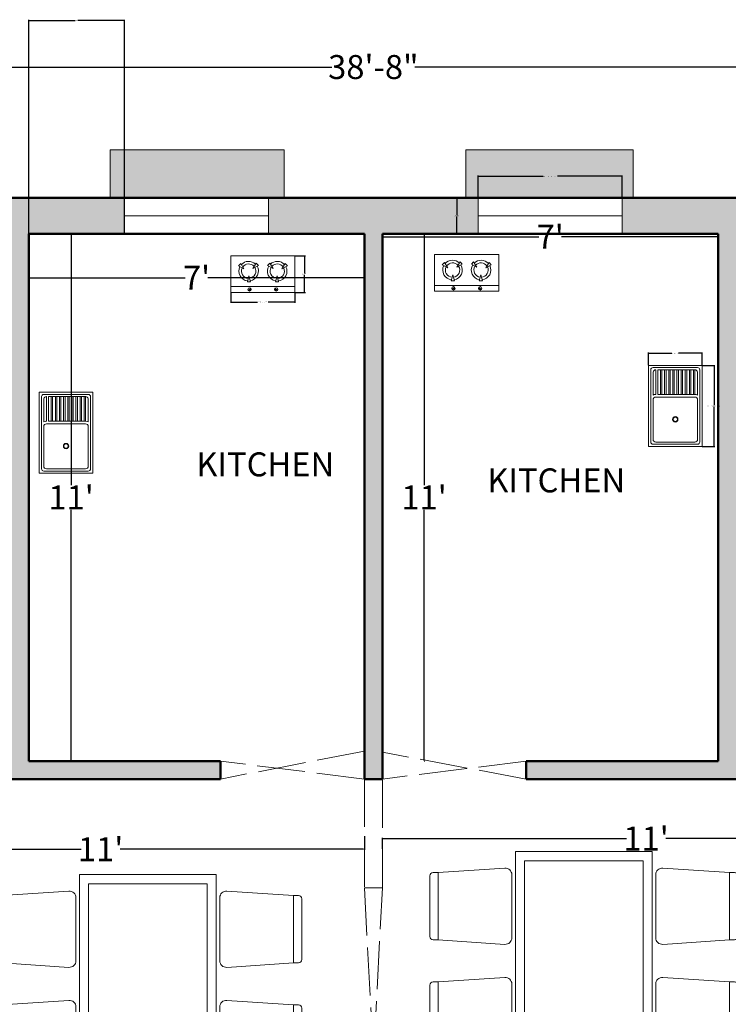
# Model space of a CAD drawing. Units: inches. Extents: x -28 to 544, y -640 to 52.
# Tile 8 of 11: x 160 to 338, y -194 to 52. Entities that reach past the tile are written whole.
import ezdxf

# ---------------------------------------------------------------- set-up
doc = ezdxf.new("R2010")
doc.units = ezdxf.units.IN
doc.header["$MEASUREMENT"] = 0
doc.linetypes.add('ACAD_ISO02W100', pattern=[15, 12, -3])
for name, color, linetype, lineweight in [('A-ANNO-DIMS', 2, 'Continuous', 18), ('A-AREA-IDEN', 7, 'Continuous', 25), ('A-EQPM', 8, 'Continuous', 18), ('A-FLOR-FIXT', 9, 'Continuous', 20), ('A-FURN', 8, 'Continuous', 18), ('A-GLAZ', 4, 'Continuous', 20), ('A-ROOF', 8, 'Continuous', 18), ('A-ROOF-PATT', 252, 'Continuous', 13), ('A-WALL', 7, 'Continuous', 50), ('A-WALL-OVHD', 8, 'ACAD_ISO02W100', 18), ('A-WALL-PATT', 5, 'Continuous', 13)]:
    doc.layers.add(name, color=color, linetype=linetype, lineweight=lineweight)
doc.styles.get("Standard").update_dxf_attribs({"font": 'arial.ttf'})
doc.dimstyles.get("Standard").update_dxf_attribs({"dimtxt": 0.18, "dimasz": 0.18, "dimexe": 0.18, "dimexo": 0.0625, "dimgap": 0.09, "dimtad": 0, "dimtih": 1, "dimtoh": 1, "dimdec": 0, "dimzin": 0, "dimdsep": 46, "dimlunit": 3, "dimtxsty": 'Standard', "dimcen": 0.09, "dimadec": 0, "dimazin": 0, "dimtfac": 1, "dimtdec": 0, "dimtofl": 0, "dimtmove": 0, "dimatfit": 3, "dimfxl": 1, "dimtolj": 1, "dimtzin": 0, "dimarcsym": 0})

# ---------------------------------------------------------------- blocks, each defined once
blk = doc.blocks.new('*D3')
at = {"layer": 'A-ANNO-DIMS', "color": 0, "lineweight": -2, "transparency": 16777216}
for p, q in [((173.13, -1.24), (172.89, -1.24)), ((173.07, -1.42), (173.07, -64.14)), ((173.07, -133.06), (173.07, -70.34)), ((173.13, -133.24), (172.89, -133.24))]:
    blk.add_line(p, q, dxfattribs=at)
at = {"layer": 'A-ANNO-DIMS', "color": 0, "transparency": 16777216}
for points in [[(173.04, -1.42), (173.1, -1.42), (173.07, -1.24)], [(173.04, -133.06), (173.1, -133.06), (173.07, -133.24)]]:
    blk.add_solid(points, dxfattribs=at)
at = {"layer": 'Defpoints', "color": 0, "transparency": 16777216}
for p in [(173.19, -1.24), (173.07, -133.24), (173.19, -133.24)]:
    blk.add_point(p, dxfattribs=at)
at = {"layer": 'A-ANNO-DIMS', "color": 0, "transparency": 16777216, "insert": (173.07, -67.24), "char_height": 6, "attachment_point": 5}
blk.add_mtext("\\A1;11'", dxfattribs=at)
blk = doc.blocks.new('*D4')
at = {"layer": 'A-ANNO-DIMS', "color": 0, "lineweight": -2, "transparency": 16777216}
for p, q in [((162.44, -12.17), (162.44, -12.06)), ((162.62, -12.24), (201.62, -12.24)), ((246.26, -12.24), (207.27, -12.24)), ((246.44, -12.17), (246.44, -12.06))]:
    blk.add_line(p, q, dxfattribs=at)
at = {"layer": 'A-ANNO-DIMS', "color": 0, "transparency": 16777216}
for points in [[(162.62, -12.21), (162.62, -12.27), (162.44, -12.24)], [(246.26, -12.21), (246.26, -12.27), (246.44, -12.24)]]:
    blk.add_solid(points, dxfattribs=at)
at = {"layer": 'Defpoints', "color": 0, "transparency": 16777216}
for p in [(162.44, -12.24), (246.44, -12.24), (246.44, -12.24)]:
    blk.add_point(p, dxfattribs=at)
at = {"layer": 'A-ANNO-DIMS', "color": 0, "transparency": 16777216, "insert": (204.44, -12.24), "char_height": 6, "attachment_point": 5}
blk.add_mtext("\\A1;7'", dxfattribs=at)
blk = doc.blocks.new('*D5')
at = {"layer": 'A-ANNO-DIMS', "color": 0, "lineweight": -2, "transparency": 16777216}
for p, q in [((250.94, -3.78), (250.94, -1.8)), ((251.12, -1.98), (290.12, -1.98)), ((334.76, -1.98), (295.77, -1.98)), ((334.94, -3.78), (334.94, -1.8))]:
    blk.add_line(p, q, dxfattribs=at)
at = {"layer": 'A-ANNO-DIMS', "color": 0, "transparency": 16777216}
for points in [[(251.12, -1.95), (251.12, -2.01), (250.94, -1.98)], [(334.76, -1.95), (334.76, -2.01), (334.94, -1.98)]]:
    blk.add_solid(points, dxfattribs=at)
at = {"layer": 'Defpoints', "color": 0, "transparency": 16777216}
for p in [(334.94, -1.98), (250.94, -3.84), (334.94, -3.84)]:
    blk.add_point(p, dxfattribs=at)
at = {"layer": 'A-ANNO-DIMS', "color": 0, "transparency": 16777216, "insert": (292.94, -1.98), "char_height": 6, "attachment_point": 5}
blk.add_mtext("\\A1;7'", dxfattribs=at)
blk = doc.blocks.new('*D6')
at = {"layer": 'A-ANNO-DIMS', "color": 0, "lineweight": -2, "transparency": 16777216}
for p, q in [((261.39, -1.42), (261.39, -64.14)), ((261.45, -1.24), (261.57, -1.24)), ((261.39, -133.06), (261.39, -70.34)), ((261.45, -133.24), (261.57, -133.24))]:
    blk.add_line(p, q, dxfattribs=at)
at = {"layer": 'A-ANNO-DIMS', "color": 0, "transparency": 16777216}
for points in [[(261.36, -1.42), (261.42, -1.42), (261.39, -1.24)], [(261.36, -133.06), (261.42, -133.06), (261.39, -133.24)]]:
    blk.add_solid(points, dxfattribs=at)
at = {"layer": 'Defpoints', "color": 0, "transparency": 16777216}
for p in [(261.39, -1.24), (261.39, -133.24), (261.39, -133.24)]:
    blk.add_point(p, dxfattribs=at)
at = {"layer": 'A-ANNO-DIMS', "color": 0, "transparency": 16777216, "insert": (261.39, -67.24), "char_height": 6, "attachment_point": 5}
blk.add_mtext("\\A1;11'", dxfattribs=at)
blk = doc.blocks.new('М12 540х820')
for p, q in [((0, 540), (-820, 540)), ((-820, 540), (-820, 0)), ((-45, 517.5), (-775, 517.5)), ((0, 0), (0, 540)), ((-797.5, 495), (-797.5, 45)), ((-775, 468), (-775, 72)), ((-347.5, 495), (-748, 495)), ((-320.5, 468), (-320.5, 72)), ((-301.7, 495), (-64.8, 495)), ((-293.7, 468), (-293.7, 472.5)), ((-293.7, 468), (-45, 468)), ((-293.7, 446.6), (-45, 446.6)), ((-293.7, 419.6), (-293.7, 446.6)), ((-293.7, 419.6), (-45, 419.6)), ((-293.7, 405), (-45, 405)), ((-293.7, 378), (-293.7, 405)), ((-45, 469.5), (-45, 468)), ((-45, 419.6), (-45, 446.6)), ((-45, 378), (-45, 405)), ((-22.5, 45), (-22.5, 495)), ((-293.7, 378), (-45, 378)), ((-293.7, 336.4), (-293.7, 363.4)), ((-293.7, 363.4), (-45, 363.4)), ((-293.7, 336.4), (-45, 336.4)), ((-293.7, 294.7), (-293.7, 321.7)), ((-293.7, 321.7), (-45, 321.7)), ((-45, 336.4), (-45, 363.4)), ((-45, 294.7), (-45, 321.7)), ((-293.7, 294.7), (-45, 294.7)), ((-293.7, 253.1), (-293.7, 280.1)), ((-293.7, 280.1), (-45, 280.1)), ((-293.7, 253.1), (-45, 253.1)), ((-293.7, 211.5), (-293.7, 238.5)), ((-293.7, 238.5), (-45, 238.5)), ((-293.7, 211.5), (-45, 211.5)), ((-45, 253.1), (-45, 280.1)), ((-45, 211.5), (-45, 238.5)), ((-293.7, 169.9), (-293.7, 196.9)), ((-293.7, 196.9), (-45, 196.9)), ((-293.7, 169.9), (-45, 169.9)), ((-293.7, 128.2), (-293.7, 155.2)), ((-293.7, 155.2), (-45, 155.2)), ((-293.7, 128.2), (-45, 128.2)), ((-293.7, 113.6), (-45, 113.6)), ((-293.7, 86.6), (-293.7, 113.6)), ((-45, 169.9), (-45, 196.9)), ((-45, 128.2), (-45, 155.2)), ((-45, 86.6), (-45, 113.6)), ((-820, 0), (0, 0)), ((-775, 22.5), (-45, 22.5)), ((-748, 45), (-347.5, 45)), ((-301.7, 45), (-64.8, 45)), ((-293.7, 86.6), (-45, 86.6)), ((-293.7, 72), (-45, 72)), ((-45, 70.5), (-45, 72))]:
    blk.add_line(p, q)
at = {"ltscale": 0.06}
for p, q in [((-820, 0), (-820, 540)), ((-820, 540), (0, 540)), ((0, 540), (0, 536.9)), ((0, 536.9), (0, 0)), ((-293.7, 446.6), (-45, 446.6)), ((-293.7, 405), (-293.7, 446.6)), ((-293.7, 363.4), (-293.7, 405)), ((-45, 446.6), (-45, 419.6)), ((-45, 419.6), (-45, 378)), ((-293.7, 321.7), (-293.7, 363.4)), ((-293.7, 280.1), (-293.7, 321.7)), ((-45, 378), (-45, 336.4)), ((-45, 336.4), (-45, 294.7)), ((-293.7, 238.5), (-293.7, 280.1)), ((-293.7, 196.9), (-293.7, 238.5)), ((-45, 294.7), (-45, 253.1)), ((-45, 253.1), (-45, 211.5)), ((-45, 211.5), (-45, 169.9)), ((-293.7, 155.2), (-293.7, 196.9)), ((-293.7, 113.6), (-293.7, 155.2)), ((-293.7, 72), (-293.7, 113.6)), ((-45, 169.9), (-45, 128.2)), ((-45, 128.2), (-45, 86.6)), ((0, 0), (-820, 0)), ((-45, 72), (-293.7, 72)), ((-45, 86.6), (-45, 72))]:
    blk.add_line(p, q, dxfattribs=at)
at = {"extrusion": (0, 0, -1)}
for centre, major_axis, start_param, end_param in [((-775, 495), (-15.9, 15.9), -0.785398, 0.785398), ((-775, 495), (-15.9, 15.9), -0.785398, 0.785398), ((-45, 495), (-15.9, -15.9), 2.356194, 3.926991), ((-45, 495), (-15.9, -15.9), 2.356194, 3.926991), ((-748, 468), (-19.1, -19.1), 0.785398, 2.356194), ((-748, 468), (-19.1, -19.1), 0.785398, 2.356194), ((-347.5, 468), (-19.1, 19.1), 0.785398, 2.356194), ((-347.5, 468), (-19.1, 19.1), 0.785398, 2.356194), ((-343.2, 468), (-35, 35), 1.779263, 2.356194), ((-343.2, 468), (-35, 35), 1.779263, 2.356192), ((-343.2, 468), (-35, 35), 2.356192, 2.356194), ((-72.3, 468.8), (-19.3, 19.3), 1.0328, 2.38382), ((-72.3, 468.8), (-19.3, 19.3), 1.0328, 1.064673), ((-72.3, 468.8), (-19.3, 19.3), 1.064673, 2.328569), ((-72.3, 468.8), (-19.3, 19.3), 2.328569, 2.38382), ((-545.5, 270), (-19.1, -19.1), 3.926991, 10.210176), ((-545.5, 270), (-19.1, -19.1), 3.926991, 10.210176), ((-545.5, 270), (-15.9, -15.9), 3.926991, 10.210176), ((-545.5, 270), (-15.9, -15.9), 3.926991, 10.210176), ((-775, 45), (-15.9, -15.9), 5.497787, 7.068583), ((-775, 45), (-15.9, -15.9), 5.497787, 7.068583), ((-748, 72), (-19.1, 19.1), 3.926991, 5.497787), ((-748, 72), (-19.1, 19.1), 3.926991, 5.497787), ((-347.5, 72), (-19.1, -19.1), 3.926991, 5.497787), ((-347.5, 72), (-19.1, -19.1), 3.926991, 5.497787), ((-343.2, 72), (-35, -35), 3.926991, 4.503922), ((-343.2, 72), (-35, -35), 3.926991, 4.503922), ((-72.3, 71.2), (-19.3, -19.3), 3.899365, 5.250385), ((-72.3, 71.2), (-19.3, -19.3), 5.218512, 5.250385), ((-72.3, 71.2), (-19.3, -19.3), 3.954617, 5.218512), ((-72.3, 71.2), (-19.3, -19.3), 3.899365, 3.954617), ((-45, 45), (-15.9, 15.9), 2.356194, 3.926991), ((-45, 45), (-15.9, 15.9), 2.356194, 3.926991)]:
    blk.add_ellipse(centre, major_axis=major_axis, ratio=1, start_param=start_param, end_param=end_param, dxfattribs=at)
blk = doc.blocks.new('*D27')
at = {"layer": 'A-ANNO-DIMS', "color": 0, "lineweight": -2, "transparency": 16777216}
for p, q in [((16.94, 7.82), (16.94, 40.69)), ((17.12, 40.51), (238.3, 40.51)), ((480.26, 40.51), (259.09, 40.51)), ((480.44, 7.82), (480.44, 40.69))]:
    blk.add_line(p, q, dxfattribs=at)
at = {"layer": 'A-ANNO-DIMS', "color": 0, "transparency": 16777216}
for points in [[(17.12, 40.54), (17.12, 40.48), (16.94, 40.51)], [(480.26, 40.54), (480.26, 40.48), (480.44, 40.51)]]:
    blk.add_solid(points, dxfattribs=at)
at = {"layer": 'Defpoints', "color": 0, "transparency": 16777216}
for p in [(480.44, 40.51), (16.94, 7.76), (480.44, 7.76)]:
    blk.add_point(p, dxfattribs=at)
at = {"layer": 'A-ANNO-DIMS', "color": 0, "transparency": 16777216, "insert": (248.69, 40.51), "char_height": 6, "attachment_point": 5}
blk.add_mtext('\\A1;38\'-8"', dxfattribs=at)
blk = doc.blocks.new('*D37')
at = {"layer": 'A-ANNO-DIMS', "color": 0, "lineweight": -2, "transparency": 16777216}
for p, q in [((114.44, -152.03), (114.44, -155.48)), ((246.44, -152.03), (246.44, -155.48)), ((114.62, -155.3), (175.55, -155.3)), ((246.26, -155.3), (185.34, -155.3))]:
    blk.add_line(p, q, dxfattribs=at)
at = {"layer": 'A-ANNO-DIMS', "color": 0, "transparency": 16777216}
for points in [[(114.62, -155.27), (114.62, -155.33), (114.44, -155.3)], [(246.26, -155.27), (246.26, -155.33), (246.44, -155.3)]]:
    blk.add_solid(points, dxfattribs=at)
at = {"layer": 'Defpoints', "color": 0, "transparency": 16777216}
for p in [(114.44, -151.97), (246.44, -151.97), (246.44, -155.3)]:
    blk.add_point(p, dxfattribs=at)
at = {"layer": 'A-ANNO-DIMS', "color": 0, "transparency": 16777216, "insert": (180.44, -155.3), "char_height": 6, "attachment_point": 5}
blk.add_mtext("\\A1;11'", dxfattribs=at)
blk = doc.blocks.new('*D38')
at = {"layer": 'A-ANNO-DIMS', "color": 0, "lineweight": -2, "transparency": 16777216}
for p, q in [((250.94, -155.24), (250.94, -152.45)), ((251.12, -152.63), (312.05, -152.63)), ((382.76, -152.63), (321.84, -152.63)), ((382.94, -152.31), (382.94, -152.81))]:
    blk.add_line(p, q, dxfattribs=at)
at = {"layer": 'A-ANNO-DIMS', "color": 0, "transparency": 16777216}
for points in [[(251.12, -152.6), (251.12, -152.66), (250.94, -152.63)], [(382.76, -152.6), (382.76, -152.66), (382.94, -152.63)]]:
    blk.add_solid(points, dxfattribs=at)
at = {"layer": 'Defpoints', "color": 0, "transparency": 16777216}
for p in [(382.94, -152.25), (382.94, -152.63), (250.94, -155.3)]:
    blk.add_point(p, dxfattribs=at)
at = {"layer": 'A-ANNO-DIMS', "color": 0, "transparency": 16777216, "insert": (316.94, -152.63), "char_height": 6, "attachment_point": 5}
blk.add_mtext("\\A1;11'", dxfattribs=at)
blk = doc.blocks.new('DINING-SET-4')
for p, q in [((0.82, 49.45), (2.05, 49.45)), ((18.79, 50.59), (2.05, 49.45)), ((2.05, 32.63), (2.05, 49.45)), ((58.27, 50.59), (75.01, 49.45)), ((76.24, 49.45), (75.01, 49.45)), ((75.01, 32.63), (75.01, 49.45)), ((0, 33.45), (0, 48.63)), ((20.52, 48.95), (20.52, 33.13)), ((56.54, 48.95), (56.54, 33.13)), ((77.06, 33.45), (77.06, 48.63)), ((2.05, 32.63), (0.82, 32.63)), ((2.05, 32.63), (18.79, 31.49)), ((75.01, 32.63), (58.27, 31.49)), ((75.01, 32.63), (76.24, 32.63)), ((2.05, 22.09), (18.79, 23.23)), ((75.01, 22.09), (58.27, 23.23)), ((0, 21.27), (0, 6.09)), ((2.05, 22.09), (0.82, 22.09)), ((2.05, 22.09), (2.05, 5.27)), ((20.52, 5.77), (20.52, 21.59)), ((56.54, 5.77), (56.54, 21.59)), ((75.01, 22.09), (76.24, 22.09)), ((75.01, 22.09), (75.01, 5.27)), ((77.06, 21.27), (77.06, 6.09)), ((0.82, 5.27), (2.05, 5.27)), ((18.79, 4.13), (2.05, 5.27)), ((58.27, 4.13), (75.01, 5.27)), ((76.24, 5.27), (75.01, 5.27))]:
    blk.add_line(p, q)
for points in [[(55.63, 0), (21.43, 0), (21.43, 54.72), (55.63, 54.72)], [(53.35, 2.28), (23.71, 2.28), (23.71, 52.44), (53.35, 52.44)]]:
    blk.add_lwpolyline(points, close=True)
for centre, radius, start, end in [((0.82, 48.63), 0.821, 90, 180), ((18.88, 48.95), 1.64, 0, 93.1221), ((58.18, 48.95), 1.64, 86.8779, 180), ((76.24, 48.63), 0.821, 0, 90), ((0.82, 33.45), 0.821, 180, 270), ((18.88, 33.13), 1.64, 266.8779, 0), ((58.18, 33.13), 1.64, 180, 273.1221), ((76.24, 33.45), 0.821, 270, 0), ((18.88, 21.59), 1.64, 0, 93.1221), ((58.18, 21.59), 1.64, 86.8779, 180), ((0.82, 21.27), 0.821, 90, 180), ((76.24, 21.27), 0.821, 0, 90), ((0.82, 6.09), 0.821, 180, 270), ((18.88, 5.77), 1.64, 266.8779, 0), ((58.18, 5.77), 1.64, 180, 273.1221), ((76.24, 6.09), 0.821, 270, 0)]:
    blk.add_arc(centre, radius, start, end)
blk = doc.blocks.new('COOKTOP-2-BURNER')
for p, q in [((2.49, 7.2), (1.93, 6.63)), ((1.93, 6.63), (3.3, 5.87)), ((3.3, 5.87), (2.49, 7.2)), ((6.37, 7.34), (5.54, 6.01)), ((5.54, 6.01), (6.91, 6.76)), ((6.91, 6.76), (6.37, 7.34)), ((9.22, 6.76), (9.76, 7.34)), ((10.59, 6.01), (9.22, 6.76)), ((9.76, 7.34), (10.59, 6.01)), ((12.82, 5.87), (13.64, 7.2)), ((14.19, 6.63), (12.82, 5.87)), ((13.64, 7.2), (14.19, 6.63)), ((4.54, 4.16), (4.16, 2.65)), ((4.16, 2.65), (4.96, 2.65)), ((4.96, 2.65), (4.54, 4.16)), ((11.17, 2.65), (11.58, 4.16)), ((11.96, 2.65), (11.17, 2.65)), ((11.58, 4.16), (11.96, 2.65)), ((16.08, 1.49), (0, 1.49))]:
    blk.add_line(p, q)
at = {"ltscale": 20}
for p, q in [((5.02, 1.04), (4.42, 0.45)), ((4.72, 0.32), (5.02, 1.04)), ((11.07, 1.04), (11.67, 0.45)), ((11.37, 0.32), (11.07, 1.04))]:
    blk.add_line(p, q, dxfattribs=at)
blk.add_lwpolyline([(0, 9.19), (16.08, 9.19), (16.08, 0), (0, 0)], close=True)
for centre in [(4.72, 0.74), (11.37, 0.74)]:
    blk.add_circle(centre, 0.423, dxfattribs=at)
for centre, radius, start, end in [((4.49, 5.32), 2.45, 45.8373, 138.7775), ((11.63, 5.32), 2.45, 41.2225, 134.1627), ((4.49, 5.32), 2.45, 153.231, 263.5995), ((4.49, 5.32), 1.8, 154.0793, 266.4247), ((4.49, 5.32), 1.8, 41.1973, 145.4439), ((4.49, 5.32), 1.8, 276.98, 32.0222), ((4.49, 5.32), 2.45, 279.2438, 31.147), ((11.63, 5.32), 2.45, 148.853, 260.7562), ((11.63, 5.32), 1.8, 147.9778, 263.02), ((11.63, 5.32), 1.8, 34.5561, 138.8027), ((11.63, 5.32), 1.8, 273.5753, 25.9207), ((11.63, 5.32), 2.45, 276.4005, 26.769)]:
    blk.add_arc(centre, radius, start, end)
blk = doc.blocks.new('WIN-36IN')
for p, q in [((0, 9), (36, 9)), ((0, 0), (0, 9)), ((36, 9), (36, 0)), ((0, 4.5), (36, 4.5)), ((36, 0), (0, 0))]:
    blk.add_line(p, q)
blk = doc.blocks.new('*D63')
at = {"layer": 'A-ANNO-DIMS', "color": 0, "lineweight": -2, "transparency": 16777216}
for p, q in [((330.99, -34.18), (334.15, -34.18)), ((333.97, -34.36), (333.97, -44.15)), ((333.97, -54.31), (333.97, -44.52)), ((330.99, -54.49), (334.15, -54.49))]:
    blk.add_line(p, q, dxfattribs=at)
at = {"layer": 'A-ANNO-DIMS', "color": 0, "transparency": 16777216}
for points in [[(333.94, -34.36), (334, -34.36), (333.97, -34.18)], [(333.94, -54.31), (334, -54.31), (333.97, -54.49)]]:
    blk.add_solid(points, dxfattribs=at)
at = {"layer": 'Defpoints', "color": 0, "transparency": 16777216}
for p in [(330.93, -34.18), (333.97, -34.18), (330.93, -54.49)]:
    blk.add_point(p, dxfattribs=at)
at = {"layer": 'A-ANNO-DIMS', "color": 0, "transparency": 16777216, "insert": (333.97, -44.33), "char_height": 0.18, "attachment_point": 5}
blk.add_mtext('\\A1;KITCHEN SINK 1\'-8 1/2" TYP.', dxfattribs=at)
blk = doc.blocks.new('*D64')
at = {"layer": 'A-ANNO-DIMS', "color": 0, "lineweight": -2, "transparency": 16777216}
for p, q in [((317.56, -34.12), (317.56, -30.96)), ((317.74, -31.14), (323.4, -31.14)), ((330.75, -31.14), (325.08, -31.14)), ((330.93, -34.12), (330.93, -30.96))]:
    blk.add_line(p, q, dxfattribs=at)
at = {"layer": 'A-ANNO-DIMS', "color": 0, "transparency": 16777216}
for points in [[(317.74, -31.11), (317.74, -31.17), (317.56, -31.14)], [(330.75, -31.11), (330.75, -31.17), (330.93, -31.14)]]:
    blk.add_solid(points, dxfattribs=at)
at = {"layer": 'Defpoints', "color": 0, "transparency": 16777216}
for p in [(317.56, -31.14), (317.56, -34.18), (330.93, -34.18)]:
    blk.add_point(p, dxfattribs=at)
at = {"layer": 'A-ANNO-DIMS', "color": 0, "transparency": 16777216, "insert": (324.24, -31.14), "char_height": 0.18, "attachment_point": 5}
blk.add_mtext('\\A1;1\'-1 1/2" TYP.', dxfattribs=at)
blk = doc.blocks.new('*D73')
at = {"layer": 'A-ANNO-DIMS', "color": 0, "lineweight": -2, "transparency": 16777216}
for p, q in [((212.99, -15.98), (212.99, -18.51)), ((229.08, -15.98), (229.08, -18.51)), ((213.17, -18.33), (219.74, -18.33)), ((228.9, -18.33), (222.34, -18.33))]:
    blk.add_line(p, q, dxfattribs=at)
at = {"layer": 'A-ANNO-DIMS', "color": 0, "transparency": 16777216}
for points in [[(213.17, -18.3), (213.17, -18.36), (212.99, -18.33)], [(228.9, -18.3), (228.9, -18.36), (229.08, -18.33)]]:
    blk.add_solid(points, dxfattribs=at)
at = {"layer": 'Defpoints', "color": 0, "transparency": 16777216}
for p in [(212.99, -15.91), (229.08, -15.91), (229.08, -18.33)]:
    blk.add_point(p, dxfattribs=at)
at = {"layer": 'A-ANNO-DIMS', "color": 0, "transparency": 16777216, "insert": (221.04, -18.33), "char_height": 0.18, "attachment_point": 5}
blk.add_mtext('\\A1;COOKTOP 1\'-4" TYP.', dxfattribs=at)
blk = doc.blocks.new('*D74')
at = {"layer": 'A-ANNO-DIMS', "color": 0, "lineweight": -2, "transparency": 16777216}
for p, q in [((229.14, -6.72), (231.67, -6.72)), ((231.49, -6.9), (231.49, -11.14)), ((231.49, -15.73), (231.49, -11.5)), ((229.14, -15.91), (231.67, -15.91))]:
    blk.add_line(p, q, dxfattribs=at)
at = {"layer": 'A-ANNO-DIMS', "color": 0, "transparency": 16777216}
for points in [[(231.46, -6.9), (231.52, -6.9), (231.49, -6.72)], [(231.46, -15.73), (231.52, -15.73), (231.49, -15.91)]]:
    blk.add_solid(points, dxfattribs=at)
at = {"layer": 'Defpoints', "color": 0, "transparency": 16777216}
for p in [(229.08, -6.72), (231.49, -6.72), (229.08, -15.91)]:
    blk.add_point(p, dxfattribs=at)
at = {"layer": 'A-ANNO-DIMS', "color": 0, "transparency": 16777216, "insert": (231.49, -11.32), "char_height": 0.18, "attachment_point": 5}
blk.add_mtext('\\A1;0\'-9" TYP.', dxfattribs=at)
blk = doc.blocks.new('*D77')
at = {"layer": 'A-ANNO-DIMS', "color": 0, "lineweight": -2, "transparency": 16777216}
for p, q in [((274.94, 7.82), (274.94, 13.34)), ((275.12, 13.16), (291.14, 13.16)), ((310.76, 13.16), (294.75, 13.16)), ((310.94, 7.82), (310.94, 13.34))]:
    blk.add_line(p, q, dxfattribs=at)
at = {"layer": 'A-ANNO-DIMS', "color": 0, "transparency": 16777216}
for points in [[(275.12, 13.19), (275.12, 13.13), (274.94, 13.16)], [(310.76, 13.19), (310.76, 13.13), (310.94, 13.16)]]:
    blk.add_solid(points, dxfattribs=at)
at = {"layer": 'Defpoints', "color": 0, "transparency": 16777216}
for p in [(310.94, 13.16), (274.94, 7.76), (310.94, 7.76)]:
    blk.add_point(p, dxfattribs=at)
at = {"layer": 'A-ANNO-DIMS', "color": 0, "transparency": 16777216, "insert": (292.94, 13.16), "char_height": 0.18, "attachment_point": 5}
blk.add_mtext('\\A1;KITCHEN WINDOW 3\'-0" TYP.', dxfattribs=at)
blk = doc.blocks.new('*D78')
at = {"layer": 'A-ANNO-DIMS', "color": 0, "lineweight": -2, "transparency": 16777216}
for p, q in [((274.88, 7.76), (269.36, 7.76)), ((269.54, 7.58), (269.54, 3.44)), ((269.54, -1.06), (269.54, 3.08)), ((274.88, -1.24), (269.36, -1.24))]:
    blk.add_line(p, q, dxfattribs=at)
at = {"layer": 'A-ANNO-DIMS', "color": 0, "transparency": 16777216}
for points in [[(269.51, 7.58), (269.57, 7.58), (269.54, 7.76)], [(269.51, -1.06), (269.57, -1.06), (269.54, -1.24)]]:
    blk.add_solid(points, dxfattribs=at)
at = {"layer": 'Defpoints', "color": 0, "transparency": 16777216}
for p in [(269.54, 7.76), (274.94, 7.76), (274.94, -1.24)]:
    blk.add_point(p, dxfattribs=at)
at = {"layer": 'A-ANNO-DIMS', "color": 0, "transparency": 16777216, "insert": (269.54, 3.26), "char_height": 0.18, "attachment_point": 5}
blk.add_mtext('\\A1;0\'-9" TYP.', dxfattribs=at)
blk = doc.blocks.new('*D87')
at = {"layer": 'A-ANNO-DIMS', "color": 0, "lineweight": -2, "transparency": 16777216}
for p, q in [((162.44, -1.18), (162.44, 52.36)), ((162.62, 52.18), (174.11, 52.18)), ((186.26, 52.18), (174.78, 52.18)), ((186.44, -1.18), (186.44, 52.36))]:
    blk.add_line(p, q, dxfattribs=at)
at = {"layer": 'A-ANNO-DIMS', "color": 0, "transparency": 16777216}
for points in [[(162.62, 52.21), (162.62, 52.15), (162.44, 52.18)], [(186.26, 52.21), (186.26, 52.15), (186.44, 52.18)]]:
    blk.add_solid(points, dxfattribs=at)
at = {"layer": 'Defpoints', "color": 0, "transparency": 16777216}
for p in [(186.44, 52.18), (162.44, -1.24), (186.44, -1.24)]:
    blk.add_point(p, dxfattribs=at)
at = {"layer": 'A-ANNO-DIMS', "color": 0, "transparency": 16777216, "insert": (174.44, 52.18), "char_height": 0.18, "attachment_point": 5}
blk.add_mtext('\\A1;2\'-0"', dxfattribs=at)

msp = doc.modelspace()

# ---------------------------------------------------------------- hatches: boundary and pattern name
at = {"layer": 'A-ROOF-PATT'}
h = msp.add_hatch(color=256, dxfattribs=at)
h.dxf.hatch_style = 1
h.set_gradient(color1=(241, 235, 31), color2=(248, 153, 30))
h.paths.add_polyline_path([(124.53, 19.76), (58.75, 19.76), (58.75, 7.76), (124.53, 7.76)])
h.paths.add_polyline_path([(226.33, 19.76), (182.83, 19.76), (182.83, 7.76), (226.33, 7.76)])
h.paths.add_polyline_path([(313.67, 19.76), (271.84, 19.76), (271.84, 7.76), (313.67, 7.76)])
h.paths.add_polyline_path([(440.55, 19.76), (372.16, 19.76), (372.16, 7.76), (440.55, 7.76)])
h.paths.add_polyline_path([(492.44, -34.91), (480.44, -34.91), (480.44, -100.18), (492.44, -100.18)])
h.paths.add_polyline_path([(492.44, -151.37), (480.44, -151.37), (480.44, -179.02), (492.44, -179.02)])
h.paths.add_polyline_path([(492.44, -207.96), (480.44, -207.96), (480.44, -238.77), (492.44, -238.77)])
h.paths.add_polyline_path([(492.44, -289.99), (480.44, -289.99), (480.44, -354.53), (492.44, -354.53)])
h.paths.add_polyline_path([(492.44, -399.27), (480.44, -399.27), (480.44, -430), (492.44, -430)])
h.paths.add_polyline_path([(492.44, -475.99), (480.44, -475.99), (480.44, -546.14), (492.44, -546.14)])
h.paths.add_polyline_path([(442.7, -587.74), (368.43, -587.74), (368.43, -599.74), (442.7, -599.74)])
h.paths.add_polyline_path([(127.64, -587.74), (54.75, -587.74), (54.75, -599.74), (127.64, -599.74)])
h.paths.add_polyline_path([(16.94, -477.43), (4.94, -477.43), (4.94, -547.54), (16.94, -547.54)])
h.paths.add_polyline_path([(16.94, -399.8), (4.94, -399.8), (4.94, -430.58), (16.94, -430.58)])
h.paths.add_polyline_path([(16.94, -287.93), (4.94, -287.93), (4.94, -356.82), (16.94, -356.82)])
h.paths.add_polyline_path([(16.94, -208.93), (4.94, -208.93), (4.94, -240.18), (16.94, -240.18)])
h.paths.add_polyline_path([(16.94, -150), (4.94, -150), (4.94, -180.17), (16.94, -180.17)])
h.paths.add_polyline_path([(16.94, -32.89), (4.94, -32.89), (4.94, -101.73), (16.94, -101.73)])
at = {"layer": 'A-WALL-PATT'}
h = msp.add_hatch(color=256, dxfattribs=at)
h.dxf.hatch_style = 1
h.paths.add_polyline_path([(25.94, -235.24), (16.94, -235.24), (16.94, -290.74), (25.94, -290.74), (25.94, -254.74), (127.94, -254.74), (127.94, -252.49), (127.94, -250.24), (118.94, -250.24), (118.94, -247.24), (109.94, -247.24), (109.94, -250.24), (25.94, -250.24)])
h.paths.add_polyline_path([(114.44, -191.74), (114.44, -137.74), (126.94, -137.74), (126.94, -135.49), (126.94, -133.24), (109.94, -133.24), (109.94, -137.74), (109.94, -191.74), (25.94, -191.74), (25.94, -176.74), (16.94, -176.74), (16.94, -211.24), (25.94, -211.24), (25.94, -196.24), (109.94, -196.24), (109.94, -219.24), (114.44, -219.24), (114.44, -196.24)])
h.paths.add_polyline_path([(25.94, -350.74), (16.94, -350.74), (16.94, -403.24), (25.94, -403.24), (25.94, -391.24), (121.94, -391.24), (121.94, -403.24), (126.44, -403.24), (126.44, -391.24), (162.44, -391.24), (162.44, -250.24), (155.94, -250.24), (155.94, -254.74), (157.94, -254.74), (157.94, -386.74), (25.94, -386.74)])
h.paths.add_polyline_path([(25.94, -443.74), (157.94, -443.74), (157.94, -446.74), (162.44, -446.74), (162.44, -439.24), (126.44, -439.24), (126.44, -427.74), (121.94, -427.74), (121.94, -439.24), (25.94, -439.24), (25.94, -427.24), (16.94, -427.24), (16.94, -481.24), (25.94, -481.24)])
h.paths.add_polyline_path([(25.94, -541.24), (16.94, -541.24), (16.94, -587.74), (61.94, -587.74), (61.94, -578.74), (25.94, -578.74)])
h.paths.add_polyline_path([(162.44, -578.74), (162.44, -474.74), (160.19, -474.74), (157.94, -474.74), (157.94, -578.74), (121.94, -578.74), (121.94, -587.74), (162.44, -587.74)])
h.paths.add_polyline_path([(200.69, -578.74), (162.44, -578.74), (162.44, -587.74), (200.69, -587.74)])
h.paths.add_polyline_path([(25.94, -97.24), (16.94, -97.24), (16.94, -152.74), (25.94, -152.74), (25.94, -137.74), (81.94, -137.74), (81.94, -135.49), (81.94, -133.24), (25.94, -133.24)])
h.paths.add_polyline_path([(210.44, -133.24), (162.44, -133.24), (162.44, -1.24), (186.44, -1.24), (186.44, 7.76), (121.94, 7.76), (121.94, -1.24), (157.94, -1.24), (157.94, -133.24), (154.94, -133.24), (154.94, -137.74), (210.44, -137.74)])
h.paths.add_polyline_path([(61.94, 7.76), (16.94, 7.76), (16.94, -37.24), (25.94, -37.24), (25.94, -1.24), (61.94, -1.24)])
h = msp.add_hatch(color=256, dxfattribs=at)
h.dxf.hatch_style = 1
h.paths.add_polyline_path([(250.94, -1.24), (274.94, -1.24), (274.94, 7.76), (222.44, 7.76), (222.44, -1.24), (246.44, -1.24), (246.44, -137.74), (250.94, -137.74)])
h = msp.add_hatch(color=256, dxfattribs=at)
h.dxf.hatch_style = 1
h.paths.add_polyline_path([(375.44, 7.76), (310.94, 7.76), (310.94, -1.24), (334.94, -1.24), (334.94, -133.24), (286.94, -133.24), (286.94, -137.74), (342.44, -137.74), (342.44, -133.24), (339.44, -133.24), (339.44, -1.24), (375.44, -1.24)])
h.paths.add_polyline_path([(480.44, 7.76), (435.44, 7.76), (435.44, -1.24), (471.44, -1.24), (471.44, -37.24), (480.44, -37.24)])
h.paths.add_polyline_path([(480.44, -97.24), (471.44, -97.24), (471.44, -133.24), (417.44, -133.24), (417.44, -135.49), (417.44, -137.74), (471.44, -137.74), (471.44, -152.74), (480.44, -152.74)])
h.paths.add_polyline_path([(480.44, -176.74), (471.44, -176.74), (471.44, -191.74), (387.44, -191.74), (387.44, -137.74), (389.44, -137.74), (389.44, -133.24), (370.44, -133.24), (370.44, -135.49), (370.44, -137.74), (382.94, -137.74), (382.94, -191.74), (382.94, -196.24), (382.94, -220.24), (385.19, -220.24), (387.44, -220.24), (387.44, -196.24), (471.44, -196.24), (471.44, -211.24), (480.44, -211.24)])
h.paths.add_polyline_path([(480.44, -235.24), (471.44, -235.24), (471.44, -250.24), (387.44, -250.24), (387.44, -248.24), (382.94, -248.24), (382.94, -250.24), (369.44, -250.24), (369.44, -252.49), (369.44, -254.74), (471.44, -254.74), (471.44, -290.74), (480.44, -290.74)])
h.paths.add_polyline_path([(480.44, -350.74), (471.44, -350.74), (471.44, -386.74), (339.44, -386.74), (339.44, -254.74), (341.44, -254.74), (341.44, -250.24), (334.94, -250.24), (334.94, -391.24), (471.44, -391.24), (471.44, -403.24), (480.44, -403.24)])
h.paths.add_polyline_path([(480.44, -427.24), (471.44, -427.24), (471.44, -439.24), (334.94, -439.24), (334.94, -446.74), (339.44, -446.74), (339.44, -443.74), (471.44, -443.74), (471.44, -481.24), (480.44, -481.24)])
h.paths.add_polyline_path([(480.44, -541.24), (471.44, -541.24), (471.44, -578.74), (435.44, -578.74), (435.44, -587.74), (480.44, -587.74)])
h.paths.add_polyline_path([(375.44, -578.74), (339.44, -578.74), (339.44, -474.74), (337.19, -474.74), (334.94, -474.74), (334.94, -578.74), (296.69, -578.74), (296.69, -587.74), (375.44, -587.74)])

# ---------------------------------------------------------------- linework, layer by layer
at = {"layer": 'A-ROOF'}
for p, q in [((182.83, 7.76), (182.83, 19.76)), ((182.83, 19.76), (226.33, 19.76)), ((226.33, 19.76), (226.33, 7.76)), ((271.84, 7.76), (271.84, 19.76)), ((271.84, 19.76), (313.67, 19.76)), ((313.67, 19.76), (313.67, 7.76))]:
    msp.add_line(p, q, dxfattribs=at)
at = {"layer": 'A-WALL'}
for p, q in [((16.94, 7.76), (480.44, 7.76)), ((162.44, -1.24), (162.44, -133.24)), ((162.44, -1.24), (246.44, -1.24)), ((246.44, -1.24), (246.44, -137.74)), ((250.94, -1.24), (250.94, -137.74)), ((250.94, -1.24), (334.94, -1.24)), ((334.94, -1.24), (334.94, -133.24)), ((162.44, -133.24), (210.44, -133.24)), ((210.44, -137.74), (210.44, -133.24)), ((286.94, -137.74), (286.94, -133.24)), ((286.94, -133.24), (334.94, -133.24)), ((154.94, -137.74), (210.44, -137.74)), ((246.44, -137.74), (250.94, -137.74)), ((286.94, -137.74), (342.44, -137.74))]:
    msp.add_line(p, q, dxfattribs=at)
at = {"layer": 'A-WALL-OVHD'}
for p, q in [((246.44, -130.77), (210.44, -137.74)), ((286.94, -137.74), (250.94, -131)), ((246.44, -137.74), (210.44, -133.24)), ((286.94, -133.24), (250.94, -137.74)), ((246.44, -137.74), (246.44, -164.95)), ((250.94, -164.95), (250.94, -137.74)), ((246.44, -164.95), (250.94, -164.95)), ((246.44, -164.95), (250.94, -250.24)), ((246.44, -250.24), (250.94, -164.95))]:
    msp.add_line(p, q, dxfattribs=at)

# ---------------------------------------------------------------- block references
at = {"layer": 'A-EQPM'}
for p in [(213, -15.91), (264.01, -15.63)]:
    msp.add_blockref('COOKTOP-2-BURNER', p, dxfattribs=at)
at = {"layer": 'A-FLOR-FIXT', "xscale": 0.0247581657147282, "yscale": 0.0247581657147282, "zscale": 0.0247581657147282, "rotation": 90}
for p in [(330.93, -34.18), (178.47, -40.88)]:
    msp.add_blockref('М12 540х820', p, dxfattribs=at)
at = {"layer": 'A-FURN'}
for p in [(262.82, -210.62), (153.73, -216.37)]:
    msp.add_blockref('DINING-SET-4', p, dxfattribs=at)
at = {"layer": 'A-GLAZ'}
for p in [(186.44, -1.24), (274.94, -1.24)]:
    msp.add_blockref('WIN-36IN', p, dxfattribs=at)

# ---------------------------------------------------------------- texts
at = {"layer": 'A-AREA-IDEN', "char_height": 6, "attachment_point": 1}
for insert in [(204.39, -55.96), (277.19, -59.97)]:
    msp.add_mtext('KITCHEN', dxfattribs=dict(at, insert=insert))

# ---------------------------------------------------------------- dimensions: what is measured, and where the dimension line sits
at = {"layer": 'A-ANNO-DIMS'}
for base, p1, p2, override, picture, middle in [((186.44, 52.18), (162.44, -1.24), (186.44, -1.24), {"dimdec": 1, "dimlfac": 1, "dimrnd": 0, "dimzin": 1, "dimdsep": 46, "dimlunit": 4, "dimfrac": 2}, '*D87', (174.44, 52.18)), ((480.44473605, 40.50985478), (16.94473605, 7.75882162), (480.44473605, 7.75882162), {"dimtxt": 6, "dimclrd": 0, "dimclre": 0, "dimclrt": 0}, '*D27', (248.69473605, 40.50985478)), ((334.94, -1.98), (250.94, -3.84), (334.94, -3.84), {"dimtxt": 6, "dimclrd": 0, "dimclre": 0, "dimclrt": 0}, '*D5', (292.94, -1.98)), ((246.44, -12.24), (162.44, -12.24), (246.44, -12.24), {"dimtxt": 6, "dimclrd": 0, "dimclre": 0, "dimclrt": 0}, '*D4', (204.44, -12.24)), ((382.94, -152.63), (250.94, -155.3), (382.94, -152.25), {"dimtxt": 6, "dimclrd": 0, "dimclre": 0, "dimclrt": 0}, '*D38', (316.94, -152.63)), ((246.44, -155.3), (114.44, -151.97), (246.44, -151.97), {"dimtxt": 6, "dimclrd": 0, "dimclre": 0, "dimclrt": 0}, '*D37', (180.44, -155.3))]:
    dim = msp.add_linear_dim(base=base, p1=p1, p2=p2, dimstyle='Standard', override=override, dxfattribs=at)
    dim.commit()
    dim.dimension.update_dxf_attribs({"geometry": picture, "text_midpoint": middle})
for base, p1, p2, text, picture, middle in [((310.94, 13.16), (274.94, 7.76), (310.94, 7.76), 'KITCHEN WINDOW <> TYP.', '*D77', (292.94, 13.16)), ((229.08, -18.33), (212.99, -15.91), (229.08, -15.91), 'COOKTOP <> TYP.', '*D73', (221.04, -18.33))]:
    dim = msp.add_linear_dim(base=base, p1=p1, p2=p2, text=text, dimstyle='Standard', override={"dimdec": 1, "dimlfac": 1, "dimrnd": 0, "dimzin": 1, "dimdsep": 46, "dimlunit": 4, "dimfrac": 2}, dxfattribs=at)
    dim.commit()
    dim.dimension.update_dxf_attribs({"geometry": picture, "text_midpoint": middle})
for base, p1, p2, angle, text, picture, middle in [((269.54, 7.76), (274.94, -1.24), (274.94, 7.76), 90, '<> TYP.', '*D78', (269.54, 3.26)), ((231.49, -6.72), (229.08, -15.91), (229.08, -6.72), 90, '<> TYP.', '*D74', (231.49, -11.32)), ((317.56, -31.14), (330.93, -34.18), (317.56, -34.18), 180, '<> TYP.', '*D64', (324.24, -31.14)), ((333.97, -34.18), (330.93, -54.49), (330.93, -34.18), 90, 'KITCHEN SINK <> TYP.', '*D63', (333.97, -44.33))]:
    dim = msp.add_linear_dim(base=base, p1=p1, p2=p2, angle=angle, text=text, dimstyle='Standard', override={"dimdec": 1, "dimlfac": 1, "dimrnd": 0, "dimzin": 1, "dimdsep": 46, "dimlunit": 4, "dimfrac": 2}, dxfattribs=at)
    dim.commit()
    dim.dimension.update_dxf_attribs({"geometry": picture, "text_midpoint": middle})
for base, p1, p2, picture, middle in [((173.07, -133.24), (173.19, -1.24), (173.19, -133.24), '*D3', (173.07, -67.24)), ((261.39, -133.24), (261.39, -1.24), (261.39, -133.24), '*D6', (261.39, -67.24))]:
    dim = msp.add_linear_dim(base=base, p1=p1, p2=p2, angle=90, dimstyle='Standard', override={"dimtxt": 6, "dimclrd": 0, "dimclre": 0, "dimclrt": 0}, dxfattribs=at)
    dim.commit()
    dim.dimension.update_dxf_attribs({"geometry": picture, "text_midpoint": middle})

doc.saveas('drawing.dxf')
